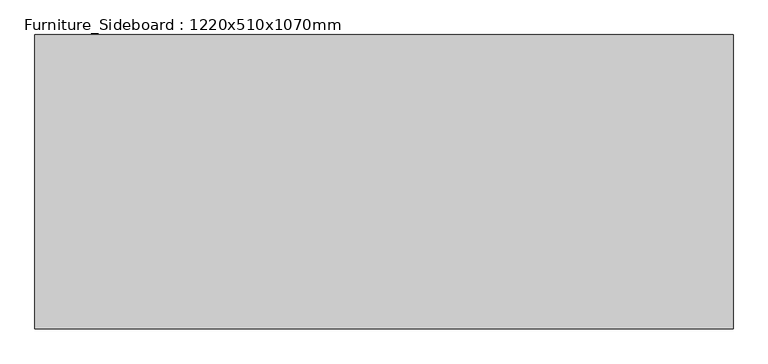
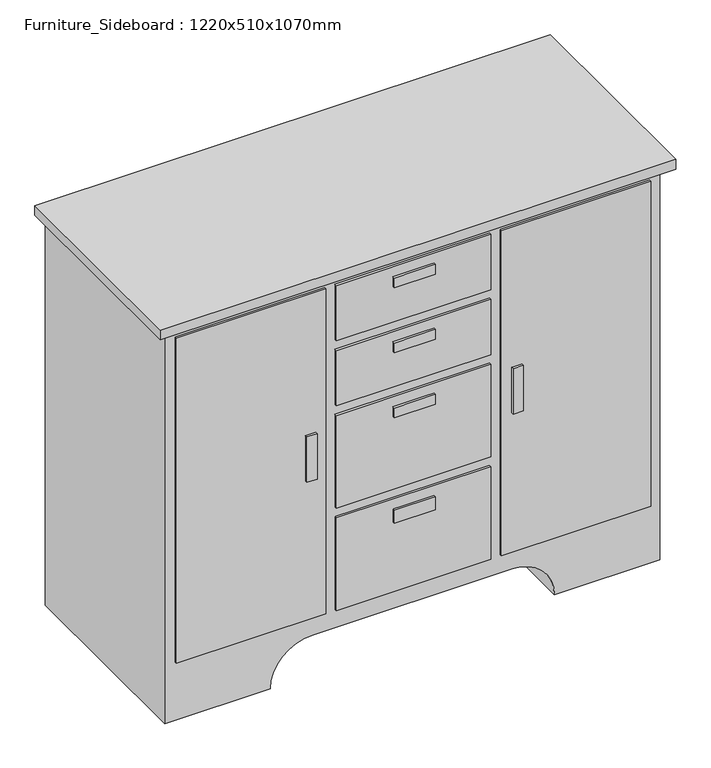
"""IFC4 building model written with IfcOpenShell, lengths in millimetres: furniture geometry, Furniture_Sideboard : 1220x510x1070mm."""

from ifc_helpers import new_model, si_unit, point, frame, frame_2d, origin, place, context, project, spatial, polyline, circle_curve, trimmed, segment, composite_curve, outline, extrude, source, transform, mapped, element, save


def furniture_sideboard_1220x510x1070mm_0243b4aa(model_context):
    return source(origin(), model_context, "Body", "SweptSolid", [
        extrude(outline(composite_curve([segment(polyline([(0.3974948, 315.4067402), (1024.9401786, 315.4067402), (1024.9401786, -904.5932598), (0.3401786, -904.5932598), (0.3401786, -644.7676781)]), True, "CONTINUOUS"), segment(trimmed(circle_curve(frame_2d((0.3401786, -541.2410879)), 103.5265902), [point((0.3401786, -644.7676781))], [point((103.8667688, -541.2410879))], True, "CARTESIAN"), True, "CONTINUOUS"), segment(polyline([(103.8667688, -541.2410879), (103.8667688, -47.5265362)]), True, "CONTINUOUS"), segment(trimmed(circle_curve(frame_2d((0.3974948, -47.5265362)), 103.469274), [point((103.8667688, -47.5265362))], [point((0.3974948, 55.9427378))], True, "CARTESIAN"), True, "CONTINUOUS"), segment(polyline([(0.3974948, 55.9427378), (0.3974948, 315.4067402)]), True, "CONTINUOUS")], self_intersect=False)), frame((0.0, -618.1629541, 0.0), z_axis=(0.0, 1.0, 0.0), x_axis=(0.0, 0.0, 1.0)), (0.0, 0.0, 1.0), 510.0),
        extrude(outline(polyline([(340.8067402, -643.5629541), (-929.9932598, -643.5629541), (-929.9932598, -108.1629541), (340.8067402, -108.1629541), (340.8067402, -643.5629541)])), frame((0.0, 0.0, 1024.9401786), z_axis=(0.0, 0.0, 1.0), x_axis=(1.0, 0.0, 0.0)), (0.0, 0.0, 1.0), 25.4),
        extrude(outline(polyline([(-510.6265932, -624.5129541), (-879.1932598, -624.5129541), (-879.1932598, -618.1629541), (-510.6265932, -618.1629541), (-510.6265932, -624.5129541)])), frame((0.0, 0.0, 152.4), z_axis=(0.0, 0.0, 1.0), x_axis=(1.0, 0.0, 0.0)), (0.0, 0.0, 1.0), 847.1401786),
        extrude(outline(polyline([(290.0067402, -624.5129541), (-78.5599265, -624.5129541), (-78.5599265, -618.1629541), (290.0067402, -618.1629541), (290.0067402, -624.5129541)])), frame((0.0, 0.0, 152.4), z_axis=(0.0, 0.0, 1.0), x_axis=(1.0, 0.0, 0.0)), (0.0, 0.0, 1.0), 847.1401786),
        extrude(outline(polyline([(-103.9599265, -624.5129541), (-485.2265932, -624.5129541), (-485.2265932, -618.1629541), (-103.9599265, -618.1629541), (-103.9599265, -624.5129541)])), frame((0.0, 0.0, 855.5121429), z_axis=(0.0, 0.0, 1.0), x_axis=(1.0, 0.0, 0.0)), (0.0, 0.0, 1.0), 144.0280357),
        extrude(outline(polyline([(-103.9599265, -624.5129541), (-485.2265932, -624.5129541), (-485.2265932, -618.1629541), (-103.9599265, -618.1629541), (-103.9599265, -624.5129541)])), frame((0.0, 0.0, 686.0841071), z_axis=(0.0, 0.0, 1.0), x_axis=(1.0, 0.0, 0.0)), (0.0, 0.0, 1.0), 144.0280357),
        extrude(outline(polyline([(-103.9599265, -624.5129541), (-485.2265932, -624.5129541), (-485.2265932, -618.1629541), (-103.9599265, -618.1629541), (-103.9599265, -624.5129541)])), frame((0.0, 0.0, 419.2420536), z_axis=(0.0, 0.0, 1.0), x_axis=(1.0, 0.0, 0.0)), (0.0, 0.0, 1.0), 241.4420536),
        extrude(outline(polyline([(-103.9599265, -624.5129541), (-485.2265932, -624.5129541), (-485.2265932, -618.1629541), (-103.9599265, -618.1629541), (-103.9599265, -624.5129541)])), frame((0.0, 0.0, 152.4), z_axis=(0.0, 0.0, 1.0), x_axis=(1.0, 0.0, 0.0)), (0.0, 0.0, 1.0), 241.4420536),
        extrude(outline(polyline([(-536.0265932, -630.8629541), (-561.4265932, -630.8629541), (-561.4265932, -624.5129541), (-536.0265932, -624.5129541), (-536.0265932, -630.8629541)])), frame((0.0, 0.0, 516.758125), z_axis=(0.0, 0.0, 1.0), x_axis=(1.0, 0.0, 0.0)), (0.0, 0.0, 1.0), 118.56),
        extrude(outline(polyline([(-244.5230145, -630.8629541), (-346.0702491, -630.8629541), (-346.0702491, -624.5129541), (-244.5230145, -624.5129541), (-244.5230145, -630.8629541)])), frame((0.0, 0.0, 948.7401786), z_axis=(0.0, 0.0, 1.0), x_axis=(1.0, 0.0, 0.0)), (0.0, 0.0, 1.0), 25.4),
        extrude(outline(polyline([(-244.5230145, -630.8629541), (-346.0702491, -630.8629541), (-346.0702491, -624.5129541), (-244.5230145, -624.5129541), (-244.5230145, -630.8629541)])), frame((0.0, 0.0, 779.3121429), z_axis=(0.0, 0.0, 1.0), x_axis=(1.0, 0.0, 0.0)), (0.0, 0.0, 1.0), 25.4),
        extrude(outline(polyline([(-244.5230145, -630.8629541), (-346.0702491, -630.8629541), (-346.0702491, -624.5129541), (-244.5230145, -624.5129541), (-244.5230145, -630.8629541)])), frame((0.0, 0.0, 609.918125), z_axis=(0.0, 0.0, 1.0), x_axis=(1.0, 0.0, 0.0)), (0.0, 0.0, 1.0), 25.4),
        extrude(outline(polyline([(-244.5230145, -630.8629541), (-346.0702491, -630.8629541), (-346.0702491, -624.5129541), (-244.5230145, -624.5129541), (-244.5230145, -630.8629541)])), frame((0.0, 0.0, 334.5620536), z_axis=(0.0, 0.0, 1.0), x_axis=(1.0, 0.0, 0.0)), (0.0, 0.0, 1.0), 33.88),
        extrude(outline(polyline([(-27.7599265, -630.8629541), (-53.1599265, -630.8629541), (-53.1599265, -624.5129541), (-27.7599265, -624.5129541), (-27.7599265, -630.8629541)])), frame((0.0, 0.0, 516.758125), z_axis=(0.0, 0.0, 1.0), x_axis=(1.0, 0.0, 0.0)), (0.0, 0.0, 1.0), 118.56),
    ])


if __name__ == "__main__":
    model = new_model("IFC4")
    model_context = context("Model", 3, world=origin())
    ifc_project = project(units=[si_unit("LENGTHUNIT", "METRE", prefix="MILLI")], contexts=[model_context])
    site = spatial("IfcSite", under=ifc_project)
    building = spatial("IfcBuilding", under=site)
    placement = place(None, origin())
    furniture_sideboard_1220x510x1070mm_shape = furniture_sideboard_1220x510x1070mm_0243b4aa(model_context)
    element("IfcFurniture", 1, ObjectType="Furniture_Sideboard : 1220x510x1070mm", at=placement, inside=building, context=model_context, shape_type="MappedRepresentation", body=[
        mapped(furniture_sideboard_1220x510x1070mm_shape, transform((0.0, 0.0, 0.0), x_axis=(1.0, 0.0, 0.0), y_axis=(0.0, 1.0, 0.0), z_axis=(0.0, 0.0, 1.0))),
    ])
    save(model, "model.ifc")

# Revit data of these elements
# Type "Furniture_Sideboard : 1220x510x1070mm"
#   Keynote = "N"
#   Depth = 1' - 8.07874"
#   Height = 3' - 5.33858"
#   Width = 4' - 0.0315"
#   Material = Wood - Cherry
#   Default Elevation = 0
#   Assembly Code = ""
# Element 1 (IfcFurniture, "Furniture_Sideboard : 1220x510x1070mm")
#   Materials on its faces: "Wood - Cherry"
# Materials
#   "Wood - Cherry": class "Wood", colour RGB 212 157 97, transparency 0
